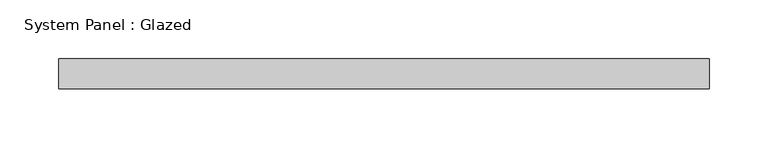
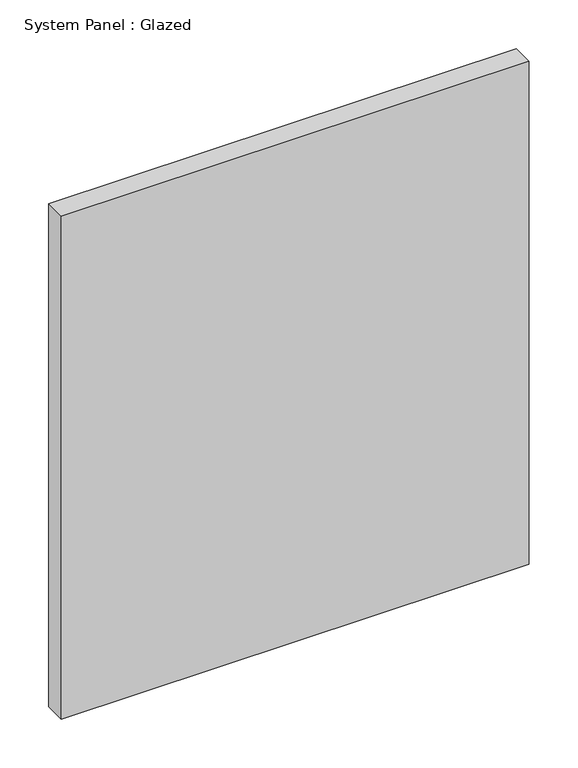
"""IFC4 building model written with IfcOpenShell, lengths in millimetres: plate geometry, System Panel : Glazed."""

from ifc_helpers import new_model, si_unit, origin, origin_with_axes, place, context, project, spatial, polyline, outline, extrude, source, transform, mapped, element, save


def system_panel_glazed_3d703fd1(model_context):
    return source(origin(), model_context, "Body", "SweptSolid", [
        extrude(outline(polyline([(276.6832607, 19.05), (-276.6832607, 19.05), (-276.6832607, 44.45), (276.6832607, 44.45), (276.6832607, 19.05)])), origin_with_axes(), (0.0, 0.0, 1.0), 628.65),
    ])


if __name__ == "__main__":
    model = new_model("IFC4")
    model_context = context("Model", 3, world=origin())
    ifc_project = project(units=[si_unit("LENGTHUNIT", "METRE", prefix="MILLI")], contexts=[model_context])
    site = spatial("IfcSite", under=ifc_project)
    building = spatial("IfcBuilding", under=site)
    placement = place(None, origin())
    system_panel_glazed_shape = system_panel_glazed_3d703fd1(model_context)
    element("IfcPlate", 1, ObjectType="System Panel : Glazed", at=placement, inside=building, context=model_context, shape_type="MappedRepresentation", body=[
        mapped(system_panel_glazed_shape, transform((0.0, 0.0, 0.0), x_axis=(1.0, 0.0, 0.0), y_axis=(0.0, 1.0, 0.0), z_axis=(0.0, 0.0, 1.0))),
    ])
    save(model, "model.ifc")

# Revit data of these elements
# Type "System Panel : Glazed"
#   Construction Type Id = "GSP4R"
#   Analytic Construction = "1/8 in Pilkington single glazing"
#   Visual Light Transmittance = 0.9
#   Solar Heat Gain Coefficient = 0.86
#   Heat Transfer Coefficient (U) = 1.18115 BTU/(h·ft²·°F)
#   Define Thermal Properties by = 1
# Element 1 (IfcPlate, "System Panel : Glazed")
#   Materials on its faces: "Glass"
# Materials
#   "Glass": class "Glass", colour RGB 0 128 192, transparency 0.75, Description = "Soda Lime Glass", Cost = 0
